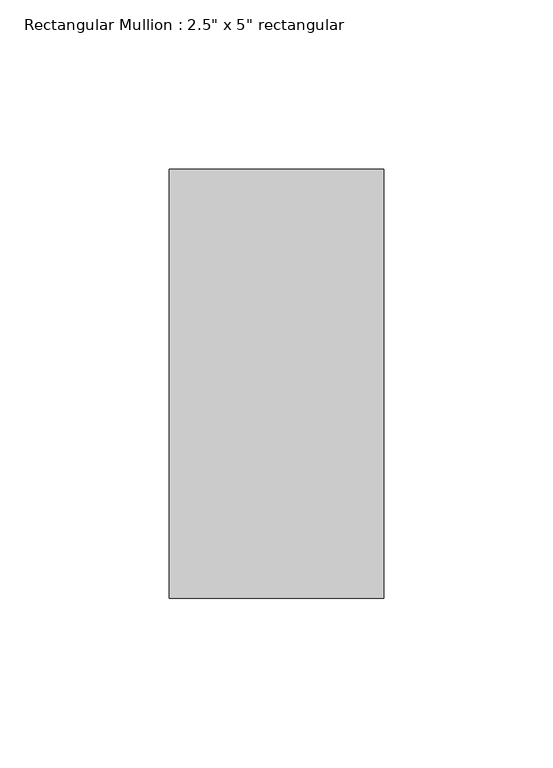
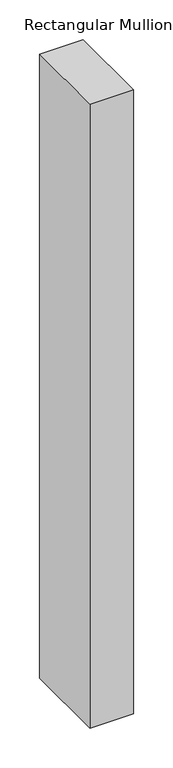
"""IFC4 building model written with IfcOpenShell, lengths in millimetres: member geometry."""

from ifc_helpers import new_model, si_unit, frame, origin, place, context, project, spatial, polyline, outline, extrude, source, transform, mapped, element, save


def member_dda01c07(model_context):
    return source(origin(), model_context, "Body", "SweptSolid", [
        extrude(outline(polyline([(31.75, 63.5), (31.75, -63.5), (-31.75, -63.5), (-31.75, 63.5), (31.75, 63.5)])), frame((0.0, 0.0, -961.0064813), z_axis=(0.0, 0.0, 1.0), x_axis=(1.0, 0.0, 0.0)), (0.0, 0.0, 1.0), 961.0064813),
    ])


if __name__ == "__main__":
    model = new_model("IFC4")
    model_context = context("Model", 3, world=origin())
    ifc_project = project(units=[si_unit("LENGTHUNIT", "METRE", prefix="MILLI")], contexts=[model_context])
    site = spatial("IfcSite", under=ifc_project)
    building = spatial("IfcBuilding", under=site)
    placement = place(None, origin())
    member_shape = member_dda01c07(model_context)
    element("IfcMember", 1, ObjectType="Rectangular Mullion : 2.5\" x 5\" rectangular", at=placement, inside=building, context=model_context, shape_type="MappedRepresentation", body=[
        mapped(member_shape, transform((0.0, 0.0, 0.0), x_axis=(1.0, 0.0, 0.0), y_axis=(0.0, 1.0, 0.0), z_axis=(0.0, 0.0, 1.0))),
    ])
    save(model, "model.ifc")

# Revit data of these elements
# Type "Rectangular Mullion : 2.5\" x 5\" rectangular"
#   built-in parameter 1007304 = 0.416667 (stored number, unit not read)
#   built-in parameter 1007301 = 0.104167 (stored number, unit not read)
#   built-in parameter 1007300 = 0.104167 (stored number, unit not read)
# Element 1 (IfcMember, "Rectangular Mullion : 2.5\" x 5\" rectangular")
#   Materials on its faces: "Aluminum"
# Materials
#   "Aluminum": class "Metal", colour RGB 247 247 247, transparency 0, Description = "Aluminum 6061", Cost = 0
